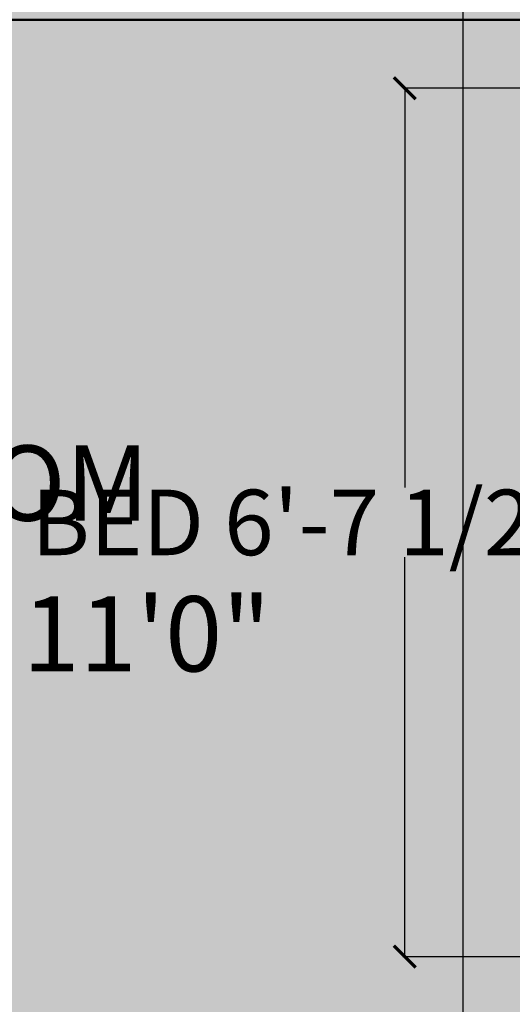
# Model space of a CAD drawing. Units: inches. Extents: x 528 to 2620, y -1066 to 798.
# Tile 27 of 41: x 1112 to 1157, y 620 to 710. Entities that reach past the tile are written whole.
import ezdxf

# ---------------------------------------------------------------- set-up
doc = ezdxf.new("R2010")
doc.units = ezdxf.units.IN
doc.header["$MEASUREMENT"] = 0
for name, color, linetype, lineweight in [('A-ANNO-DIMS', 2, 'Continuous', 18), ('A-AREA-IDEN', 7, 'Continuous', 18), ('A-WALL', 7, 'Continuous', 50), ('A-WALL-PATT', 8, 'Continuous', 13)]:
    doc.layers.add(name, color=color, linetype=linetype, lineweight=lineweight)
doc.styles.get("Standard").update_dxf_attribs({"font": 'arial.ttf'})
doc.dimstyles.get("Standard").update_dxf_attribs({"dimtxt": 6, "dimasz": 2, "dimexe": 0.18, "dimexo": 0.0625, "dimgap": 0.09, "dimtad": 0, "dimtih": 1, "dimtoh": 1, "dimdec": 1, "dimzin": 0, "dimdsep": 46, "dimlunit": 3, "dimtxsty": 'Standard', "dimblk": 'ARCHTICK', "dimcen": 0.09, "dimadec": 0, "dimazin": 0, "dimtfac": 1, "dimtdec": 1, "dimtofl": 0, "dimtmove": 0, "dimatfit": 3, "dimfxl": 1, "dimtolj": 1, "dimtzin": 0, "dimarcsym": 0})

# ---------------------------------------------------------------- blocks, each defined once
blk = doc.blocks.new('_ArchTick')
at = {"color": 0, "linetype": 'ByBlock', "const_width": 0.15}
blk.add_lwpolyline([(-0.5, -0.5), (0.5, 0.5)], dxfattribs=at)
blk = doc.blocks.new('*D42')
at = {"layer": 'A-ANNO-DIMS', "color": 0, "lineweight": -2, "transparency": 16777216}
for p, q in [((1159.521, 703.64), (1147.464, 703.64)), ((1147.644, 703.64), (1147.644, 667.032)), ((1147.644, 624.039), (1147.644, 660.647)), ((1159.521, 624.039), (1147.464, 624.039))]:
    blk.add_line(p, q, dxfattribs=at)
at = {"layer": 'Defpoints', "color": 0, "transparency": 16777216}
for p in [(1159.584, 703.64), (1147.644, 624.039), (1159.584, 624.039)]:
    blk.add_point(p, dxfattribs=at)
at = {"layer": 'A-ANNO-DIMS', "color": 0, "lineweight": -2, "transparency": 16777216, "xscale": 2, "yscale": 2, "zscale": 2}
for p, rotation in [((1147.644, 703.64), 90), ((1147.644, 624.039), 270)]:
    blk.add_blockref('_ArchTick', p, dxfattribs=dict(at, rotation=rotation))
at = {"layer": 'A-ANNO-DIMS', "color": 0, "transparency": 16777216, "insert": (1147.644, 663.839), "char_height": 6, "attachment_point": 5}
blk.add_mtext('\\A1;BED 6\'-7 1/2" TYP.', dxfattribs=at)
blk = doc.blocks.new('*D66')
at = {"layer": 'A-ANNO-DIMS', "color": 0, "lineweight": -2, "transparency": 16777216}
for p, q in [((1065.996, 400.485), (1065.996, 751.102)), ((1065.996, 750.922), (1101.456, 750.922)), ((1152.996, 750.922), (1117.537, 750.922)), ((1152.996, 400.485), (1152.996, 751.102))]:
    blk.add_line(p, q, dxfattribs=at)
at = {"layer": 'Defpoints', "color": 0, "transparency": 16777216}
for p in [(1152.996, 750.922), (1065.996, 400.422), (1152.996, 400.422)]:
    blk.add_point(p, dxfattribs=at)
at = {"layer": 'A-ANNO-DIMS', "color": 0, "lineweight": -2, "transparency": 16777216, "xscale": 2, "yscale": 2, "zscale": 2, "rotation": 180}
blk.add_blockref('_ArchTick', (1065.996, 750.922), dxfattribs=at)
at = {"layer": 'A-ANNO-DIMS', "color": 0, "lineweight": -2, "transparency": 16777216, "xscale": 2, "yscale": 2, "zscale": 2}
blk.add_blockref('_ArchTick', (1152.996, 750.922), dxfattribs=at)
at = {"layer": 'A-ANNO-DIMS', "color": 0, "transparency": 16777216, "insert": (1109.496, 750.922), "char_height": 6, "attachment_point": 5}
blk.add_mtext('\\A1;7\'-3"', dxfattribs=at)

msp = doc.modelspace()

# ---------------------------------------------------------------- hatches: boundary and pattern name
at = {"layer": 'A-WALL-PATT', "transparency": 33554521}
h = msp.add_hatch(color=256, dxfattribs=at)
h.dxf.hatch_style = 1
h.paths.add_polyline_path([(1065.996, 709.922), (1114.496, 709.922), (1114.496, 718.922), (1056.996, 718.922), (1056.996, 667.922), (1065.996, 667.922)])
h.paths.add_polyline_path([(1227.496, 718.922), (1162.496, 718.922), (1162.496, 709.922), (1210.996, 709.922), (1210.996, 577.922), (1205.418, 577.922), (1205.496, 573.422), (1210.996, 573.422), (1210.996, 567.422), (1215.496, 567.422), (1215.496, 669.422), (1267.996, 669.422), (1267.996, 675.922), (1263.496, 675.922), (1263.496, 673.922), (1215.496, 673.922), (1215.496, 709.922), (1227.496, 709.922)])
h.paths.add_polyline_path([(1344.996, 718.922), (1315.996, 718.922), (1315.996, 709.922), (1335.996, 709.922), (1335.996, 641.672), (1344.996, 641.672)])
h.paths.add_polyline_path([(1065.996, 619.922), (1056.996, 619.922), (1056.996, 561.422), (1065.996, 561.422), (1065.996, 573.422), (1160.996, 573.422), (1160.996, 569.422), (1165.496, 569.422), (1165.496, 577.922), (1065.996, 577.922)])
h.paths.add_polyline_path([(1215.996, 391.422), (1215.996, 400.422), (1206.996, 400.422), (1200.996, 400.422), (1200.996, 397.422), (1200.996, 391.422), (1206.996, 391.422), (1206.996, 268.922), (1251.996, 268.922), (1251.996, 277.922), (1215.996, 277.922), (1215.996, 359.767)])
h.paths.add_polyline_path([(1344.996, 395.922), (1335.996, 395.922), (1287.996, 395.922), (1287.996, 391.422), (1335.996, 391.422), (1335.996, 277.922), (1299.996, 277.922), (1299.996, 268.922), (1344.996, 268.922)])
h.paths.add_polyline_path([(1344.996, 593.672), (1335.996, 593.672), (1335.996, 525.422), (1215.496, 525.422), (1215.496, 527.172), (1210.996, 527.172), (1210.996, 520.922), (1335.996, 520.922), (1335.996, 443.922), (1344.996, 443.922)])
h.paths.add_polyline_path([(1065.996, 520.922), (1165.496, 520.922), (1165.496, 545.422), (1160.996, 545.422), (1160.996, 525.422), (1065.996, 525.422), (1065.996, 537.422), (1056.996, 537.422), (1056.996, 484.672), (1065.996, 484.672)])
h.paths.add_polyline_path([(1065.996, 436.672), (1056.996, 436.672), (1056.996, 391.422), (1085.496, 391.422), (1085.496, 400.422), (1065.996, 400.422)])
h.paths.add_polyline_path([(1152.996, 397.422), (1152.996, 400.422), (1133.496, 400.422), (1133.496, 391.422), (1152.996, 391.422)])
at = {"layer": 'A-WALL-PATT', "transparency": 33554681}
h = msp.add_hatch(color=256, dxfattribs=at)
h.dxf.hatch_style = 1
h.paths.add_polyline_path([(1061.996, 665.922), (1060.996, 665.922), (1060.996, 621.922), (1061.996, 621.922)])
h.paths.add_polyline_path([(1065.996, 667.922), (1056.996, 667.922), (1056.996, 665.922), (1065.996, 665.922)])
h.paths.add_polyline_path([(1065.996, 621.922), (1056.996, 621.922), (1056.996, 619.922), (1065.996, 619.922)])
h.paths.add_polyline_path([(1160.496, 714.922), (1116.496, 714.922), (1116.496, 713.922), (1160.496, 713.922)])
h.paths.add_polyline_path([(1162.496, 718.922), (1160.496, 718.922), (1160.496, 709.922), (1162.496, 709.922)])
h.paths.add_polyline_path([(1116.496, 718.922), (1114.496, 718.922), (1114.496, 709.922), (1116.496, 709.922)])
h.paths.add_polyline_path([(1251.496, 714.922), (1227.496, 714.922), (1227.496, 713.922), (1251.496, 713.922)])
h.paths.add_polyline_path([(1313.996, 714.922), (1269.996, 714.922), (1269.996, 713.922), (1313.996, 713.922)])
h.paths.add_polyline_path([(1315.996, 718.922), (1313.996, 718.922), (1313.996, 709.922), (1315.996, 709.922)])
h.paths.add_polyline_path([(1269.996, 718.922), (1267.996, 718.922), (1267.996, 709.922), (1269.996, 709.922)])
h.paths.add_polyline_path([(1087.496, 400.422), (1085.496, 400.422), (1085.496, 391.422), (1087.496, 391.422)])
h.paths.add_polyline_path([(1131.496, 396.422), (1087.496, 396.422), (1087.496, 395.422), (1131.496, 395.422)])
h.paths.add_polyline_path([(1133.496, 400.422), (1131.496, 400.422), (1131.496, 391.422), (1133.496, 391.422)])
h.paths.add_polyline_path([(1065.996, 438.672), (1056.996, 438.672), (1056.996, 436.672), (1065.996, 436.672)])
h.paths.add_polyline_path([(1065.996, 484.672), (1056.996, 484.672), (1056.996, 482.672), (1065.996, 482.672)])
h.paths.add_polyline_path([(1061.996, 482.672), (1060.996, 482.672), (1060.996, 438.672), (1061.996, 438.672)])
h = msp.add_hatch(color=256, dxfattribs=at)
h.dxf.hatch_style = 1
h.paths.add_polyline_path([(1065.996, 665.922), (1061.996, 665.922), (1061.996, 621.922), (1065.996, 621.922)])
h.paths.add_polyline_path([(1060.996, 665.922), (1056.996, 665.922), (1056.996, 621.922), (1060.996, 621.922)])
h.paths.add_polyline_path([(1160.496, 713.922), (1116.496, 713.922), (1116.496, 709.922), (1160.496, 709.922)])
h.paths.add_polyline_path([(1160.496, 718.922), (1116.496, 718.922), (1116.496, 714.922), (1160.496, 714.922)])
h.paths.add_polyline_path([(1251.496, 713.922), (1227.496, 713.922), (1227.496, 709.922), (1251.496, 709.922)])
h.paths.add_polyline_path([(1251.496, 718.922), (1227.496, 718.922), (1227.496, 714.922), (1251.496, 714.922)])
h.paths.add_polyline_path([(1313.996, 713.922), (1269.996, 713.922), (1269.996, 709.922), (1313.996, 709.922)])
h.paths.add_polyline_path([(1313.996, 718.922), (1269.996, 718.922), (1269.996, 714.922), (1313.996, 714.922)])
h.paths.add_polyline_path([(1344.996, 639.672), (1340.996, 639.672), (1340.996, 595.672), (1344.996, 595.672)])
h.paths.add_polyline_path([(1339.996, 639.672), (1335.996, 639.672), (1335.996, 595.672), (1339.996, 595.672)])
h.paths.add_polyline_path([(1344.996, 441.922), (1340.996, 441.922), (1340.996, 397.922), (1344.996, 397.922)])
h.paths.add_polyline_path([(1339.996, 441.922), (1335.996, 441.922), (1335.996, 397.922), (1339.996, 397.922)])
h.paths.add_polyline_path([(1297.996, 272.922), (1253.996, 272.922), (1253.996, 268.922), (1297.996, 268.922)])
h.paths.add_polyline_path([(1297.996, 277.922), (1253.996, 277.922), (1253.996, 273.922), (1297.996, 273.922)])
h.paths.add_polyline_path([(1131.496, 395.422), (1087.496, 395.422), (1087.496, 391.422), (1131.496, 391.422)])
h.paths.add_polyline_path([(1131.496, 400.422), (1087.496, 400.422), (1087.496, 396.422), (1131.496, 396.422)])
h.paths.add_polyline_path([(1065.996, 482.672), (1061.996, 482.672), (1061.996, 438.672), (1065.996, 438.672)])
h.paths.add_polyline_path([(1060.996, 482.672), (1056.996, 482.672), (1056.996, 438.672), (1060.996, 438.672)])
h.paths.add_polyline_path([(1065.996, 561.422), (1061.996, 561.422), (1061.996, 537.422), (1065.996, 537.422)])
h.paths.add_polyline_path([(1060.996, 561.422), (1056.996, 561.422), (1056.996, 537.422), (1060.996, 537.422)])
at = {"layer": 'A-WALL-PATT', "transparency": 33554536}
h = msp.add_hatch(color=256, dxfattribs=at)
h.dxf.hatch_style = 1
h.paths.add_polyline_path([(1335.996, 709.922), (1267.996, 709.922), (1267.996, 699.922), (1266.746, 699.922), (1266.746, 675.922), (1267.996, 675.922), (1267.996, 669.422), (1215.496, 669.422), (1215.496, 567.172), (1216.996, 567.172), (1256.996, 567.172), (1256.996, 565.422), (1256.958, 565.422, -0.401453), (1216.996, 527.172), (1215.496, 527.172), (1215.496, 525.422), (1335.996, 525.422)], flags=17)
h.paths.add_polyline_path([(1285.032, 635.927), (1285.229, 636.128), (1285.672, 636.263), (1286.206, 636.02), (1286.976, 636.084), (1332.983, 636.084), (1333.363, 636.222), (1333.82, 636.084), (1334.115, 635.714), (1334.115, 635.3), (1333.907, 634.86), (1333.82, 634.827), (1333.82, 592.738), (1333.967, 592.604), (1334.115, 592.291), (1334.115, 591.877), (1333.82, 591.507), (1333.363, 591.369), (1332.983, 591.507), (1332.638, 591.789), (1332.638, 591.507), (1286.976, 591.507), (1286.173, 591.672), (1286.066, 591.574), (1285.681, 591.37), (1285.229, 591.507), (1285.032, 591.709), (1284.834, 592.098), (1284.983, 592.537), (1285.13, 592.688), (1285.13, 634.948), (1284.983, 635.099), (1284.834, 635.537)], flags=16)
h.paths.add_polyline_path([(1285.032, 635.927), (1285.229, 636.128), (1285.672, 636.263), (1286.206, 636.02), (1286.976, 636.084), (1332.983, 636.084), (1333.363, 636.222), (1333.82, 636.084), (1334.115, 635.714), (1334.115, 635.3), (1333.967, 634.987), (1333.82, 634.853), (1333.82, 592.738), (1333.967, 592.604), (1334.115, 592.291), (1334.115, 591.877), (1333.82, 591.507), (1333.363, 591.369), (1332.983, 591.507), (1332.638, 591.789), (1332.638, 592.246), (1332.638, 635.345), (1332.638, 635.802), (1332.983, 636.084), (1312.232, 636.084), (1311.1, 635.479), (1310.632, 635.479), (1310.435, 635.233), (1309.943, 635.099), (1309.696, 634.987), (1309.056, 634.763), (1308.712, 634.607), (1308.318, 634.607), (1307.752, 634.36), (1307.112, 634.271), (1307.013, 634.114), (1306.767, 634.025), (1307.255, 633.283), (1306.866, 633.04), (1306.767, 632.884), (1306.373, 632.637), (1306.029, 632.548), (1305.536, 632.414), (1315.472, 618.494), (1316.321, 619.388), (1312.773, 622.858), (1319.616, 630.109), (1320.067, 629.676), (1320.109, 629.997), (1320.281, 630.601), (1320.527, 631.183), (1320.527, 632.011), (1320.256, 632.548), (1320.109, 633.13), (1320.06, 633.734), (1320.626, 634.025), (1321.216, 634.159), (1321.856, 634.114), (1322.447, 633.913), (1322.989, 633.622), (1324.096, 633.622), (1324.638, 633.913), (1325.229, 634.07), (1325.869, 634.07), (1326.435, 633.913), (1326.976, 633.622), (1328.355, 633.622), (1328.896, 633.913), (1329.487, 634.114), (1330.103, 634.159), (1330.693, 634.025), (1331.284, 633.734), (1331.235, 633.13), (1331.087, 632.548), (1330.792, 632.011), (1330.792, 631.183), (1331.038, 630.601), (1331.235, 629.997), (1331.284, 629.415), (1331.186, 628.788), (1331.038, 628.184), (1330.792, 627.602), (1330.792, 626.774), (1331.038, 626.193), (1331.235, 625.588), (1331.284, 625.007), (1331.186, 624.38), (1331.038, 623.776), (1330.792, 623.239), (1330.792, 622.366), (1331.038, 621.829), (1331.235, 621.247), (1331.284, 620.598), (1331.186, 619.972), (1331.038, 619.367), (1330.792, 618.83), (1330.792, 617.958), (1331.087, 617.421), (1331.235, 616.884), (1331.284, 616.235), (1331.284, 615.518), (1330.693, 615.272), (1330.103, 615.116), (1329.487, 615.116), (1328.896, 615.317), (1328.355, 615.653), (1326.976, 615.653), (1326.435, 615.317), (1325.869, 615.16), (1325.229, 615.16), (1324.638, 615.317), (1324.096, 615.653), (1323.242, 615.653), (1324.933, 614.042), (1322.978, 611.983), (1324.096, 611.983), (1324.638, 612.274), (1325.278, 612.43), (1325.869, 612.43), (1326.484, 612.274), (1327.026, 611.983), (1328.355, 611.983), (1328.896, 612.274), (1329.487, 612.475), (1330.103, 612.52), (1330.743, 612.386), (1331.284, 612.072), (1331.284, 611.356), (1331.284, 610.752), (1331.087, 610.17), (1330.792, 609.633), (1330.792, 608.805), (1331.087, 608.223), (1331.235, 607.619), (1331.284, 606.993), (1331.235, 606.411), (1331.087, 605.807), (1330.792, 605.225), (1330.792, 604.397), (1331.087, 603.815), (1331.235, 603.211), (1331.284, 602.629), (1331.235, 602.002), (1331.087, 601.398), (1330.792, 600.861), (1330.792, 599.988), (1331.087, 599.451), (1331.235, 598.87), (1331.284, 598.221), (1331.235, 597.594), (1331.087, 596.99), (1330.792, 596.453), (1330.792, 595.58), (1331.087, 595.043), (1331.284, 594.506), (1331.284, 593.857), (1330.743, 593.611), (1330.103, 593.477), (1329.487, 593.477), (1328.896, 593.678), (1328.355, 594.014), (1327.026, 594.014), (1326.484, 593.678), (1325.869, 593.521), (1325.278, 593.521), (1324.638, 593.678), (1324.096, 594.014), (1323.038, 594.014), (1322.496, 593.678), (1321.906, 593.477), (1321.266, 593.477), (1320.626, 593.611), (1320.109, 593.857), (1320.109, 594.506), (1320.281, 595.043), (1320.576, 595.58), (1320.576, 596.453), (1320.281, 596.99), (1320.158, 597.594), (1320.104, 598.015), (1319.616, 597.549), (1315.659, 601.729), (1312.232, 591.574), (1311.74, 591.664), (1311.592, 591.91), (1310.78, 592.402), (1309.549, 592.895), (1308.958, 592.895), (1308.712, 593.029), (1308.564, 593.141), (1307.752, 593.521), (1306.767, 593.611), (1307.248, 594.356), (1306.866, 594.595), (1306.373, 594.842), (1306.029, 595.088), (1305.536, 595.244), (1315.465, 609.354), (1310.927, 613.706), (1315.472, 618.494), (1305.536, 632.414), (1306.029, 632.548), (1306.373, 632.637), (1306.767, 632.884), (1306.866, 633.04), (1307.255, 633.283), (1306.767, 634.025), (1307.013, 634.114), (1307.112, 634.271), (1307.752, 634.36), (1308.318, 634.607), (1308.712, 634.607), (1309.056, 634.763), (1309.696, 634.987), (1309.943, 635.099), (1310.435, 635.233), (1310.632, 635.479), (1311.1, 635.479), (1312.232, 636.084), (1286.976, 636.084), (1286.216, 636.021), (1286.411, 635.444), (1286.213, 635.054), (1286.016, 634.853), (1285.869, 634.808), (1285.869, 592.839), (1286.153, 592.731), (1286.41, 592.188), (1286.231, 591.66), (1286.173, 591.672), (1286.066, 591.574), (1285.681, 591.37), (1285.229, 591.507), (1285.032, 591.709), (1284.834, 592.098), (1284.983, 592.537), (1285.13, 592.688), (1285.13, 634.948), (1284.983, 635.099), (1284.834, 635.537)], flags=0)
h.paths.add_polyline_path([(1322.501, 653.596), (1333.646, 653.596), (1333.646, 637.994), (1322.501, 637.994)], flags=16)
h.paths.add_polyline_path([(1323.616, 652.482), (1332.531, 652.482), (1332.531, 639.108), (1323.616, 639.108)], flags=0)
edge = h.paths.add_edge_path(flags=0)
edge.add_ellipse((1328.073, 645.795), major_axis=(2.245, 2.245), ratio=1, start_angle=405, end_angle=495, ccw=False)
edge.add_ellipse((1328.073, 645.795), major_axis=(2.245, 2.245), ratio=1, start_angle=675, end_angle=765, ccw=False)
edge.add_ellipse((1328.073, 645.795), major_axis=(2.245, 2.245), ratio=1, start_angle=585, end_angle=675, ccw=False)
edge.add_ellipse((1328.073, 645.795), major_axis=(2.245, 2.245), ratio=1, start_angle=495, end_angle=585, ccw=False)
h.paths.add_polyline_path([(1320.576, 628.386), (1320.33, 628.005), (1320.615, 628.548)], flags=0)
h.paths.add_polyline_path([(1317.893, 604.889), (1318.78, 604.643), (1319.764, 604.285), (1318.878, 604.531)], flags=0)
h.paths.add_polyline_path([(1320.33, 599.653), (1320.576, 599.25), (1320.576, 599.16)], flags=0)
h.paths.add_polyline_path([(1322.501, 589.597), (1333.646, 589.597), (1333.646, 573.995), (1322.501, 573.995)], flags=16)
h.paths.add_polyline_path([(1323.616, 588.482), (1332.531, 588.482), (1332.531, 575.109), (1323.616, 575.109)], flags=0)
edge = h.paths.add_edge_path(flags=0)
edge.add_ellipse((1328.073, 581.796), major_axis=(-2.245, 2.245), ratio=1, start_angle=-45, end_angle=45, ccw=False)
edge.add_ellipse((1328.073, 581.796), major_axis=(-2.245, 2.245), ratio=1, start_angle=-135, end_angle=-45, ccw=False)
edge.add_ellipse((1328.073, 581.796), major_axis=(-2.245, 2.245), ratio=1, start_angle=135, end_angle=-135, ccw=False)
edge.add_ellipse((1328.073, 581.796), major_axis=(-2.245, 2.245), ratio=1, start_angle=45, end_angle=135, ccw=False)
h.paths.add_polyline_path([(1264.746, 699.922), (1263.496, 699.922), (1263.496, 709.922), (1215.496, 709.922), (1215.496, 673.922), (1263.496, 673.922), (1263.496, 675.922), (1264.746, 675.922)], flags=16)
h.paths.add_polyline_path([(1162.192, 569.422), (1160.996, 569.422), (1160.996, 573.422), (1065.996, 573.422), (1065.996, 525.422), (1160.996, 525.422), (1160.996, 545.422), (1162.192, 545.422)])
h.paths.add_polyline_path([(1256.958, 565.422), (1256.996, 565.422), (1256.996, 567.172), (1216.996, 567.172), (1215.496, 567.172), (1215.496, 567.422), (1210.996, 567.422), (1210.996, 573.422), (1205.496, 573.422), (1205.418, 577.922), (1210.996, 577.922), (1210.996, 709.922), (1065.996, 709.922), (1065.996, 577.922), (1165.496, 577.922), (1165.496, 569.422), (1164.192, 569.422), (1164.192, 545.422), (1165.496, 545.422), (1165.496, 520.922), (1152.996, 520.922), (1152.996, 484.922), (1101.996, 484.922), (1101.996, 436.422), (1152.996, 436.422), (1152.996, 400.422), (1152.996, 391.422), (1200.996, 391.422), (1200.996, 400.422), (1206.996, 400.422), (1215.996, 400.422), (1215.996, 391.422), (1215.996, 277.922), (1335.996, 277.922), (1335.996, 391.422), (1287.996, 391.422), (1287.996, 395.922), (1335.996, 395.922), (1335.996, 443.922), (1335.996, 520.922), (1210.996, 520.922), (1210.996, 527.172), (1215.496, 527.172), (1216.996, 527.172, 0.401453)])
h.paths.add_polyline_path([(1167.246, 579.422), (1165.496, 579.422), (1165.496, 619.422), (1167.246, 619.422)], flags=16)
h.paths.add_polyline_path([(1227.97, 501.564), (1236.36, 502.031), (1236.36, 492.555), (1227.97, 493.021, -0.254069)], flags=16)
h.paths.add_polyline_path([(1243.336, 515.692, -0.254069), (1251.879, 515.692), (1252.345, 507.301), (1242.87, 507.301)], flags=16)
h.paths.add_polyline_path([(1239.185, 504.685), (1256.03, 504.685), (1256.03, 479.416), (1239.185, 479.416)], flags=16)
h.paths.add_polyline_path([(1227.97, 489.602), (1236.36, 490.068), (1236.36, 480.592), (1227.97, 481.058, -0.254069)], flags=16)
h.paths.add_polyline_path([(1197.201, 624.039), (1197.201, 639.641), (1208.345, 639.641), (1208.345, 624.039)], flags=16)
h.paths.add_polyline_path([(1198.315, 625.153), (1198.315, 638.526), (1207.231, 638.526), (1207.231, 625.153)], flags=0)
h.paths.add_polyline_path([(1258.855, 502.031), (1267.245, 501.564, -0.254069), (1267.245, 493.021), (1258.855, 492.555)], flags=16)
h.paths.add_polyline_path([(1271.589, 519.657), (1333.671, 519.657), (1333.671, 451.595), (1319.087, 451.595), (1319.087, 505.072), (1288.093, 505.072), (1284.447, 505.072, -0.883215), (1270.678, 514.188), (1270.678, 518.745, -0.414214)], flags=16)
h.paths.add_polyline_path([(1331.848, 517.834), (1331.848, 453.418), (1328.202, 453.418), (1328.202, 505.072), (1298.424, 505.072), (1298.424, 514.188), (1288.093, 514.188), (1288.093, 517.834)], flags=0)
h.paths.add_polyline_path([(1242.87, 476.8), (1252.345, 476.8), (1251.879, 468.409, -0.254069), (1243.336, 468.409)], flags=16)
h.paths.add_polyline_path([(1258.855, 490.068), (1267.245, 489.602, -0.254069), (1267.245, 481.058), (1258.855, 480.592)], flags=16)
h.paths.add_polyline_path([(1161.676, 641.551), (1160.873, 641.716), (1160.765, 641.618), (1160.38, 641.414), (1159.928, 641.551), (1159.731, 641.753), (1159.534, 642.142), (1159.682, 642.581), (1159.83, 642.732), (1159.83, 684.992), (1159.682, 685.143), (1159.534, 685.582), (1159.731, 685.971), (1159.928, 686.172), (1160.371, 686.307), (1160.905, 686.064), (1161.676, 686.128), (1207.682, 686.128), (1208.063, 686.266), (1208.519, 686.128), (1208.815, 685.758), (1208.815, 685.344), (1208.607, 684.904), (1208.519, 684.871), (1208.519, 642.782), (1208.667, 642.648), (1208.877, 642.201), (1208.716, 641.797), (1208.519, 641.551), (1208.063, 641.413), (1207.682, 641.551), (1207.338, 641.833), (1207.338, 641.551)], flags=16)
h.paths.add_polyline_path([(1186.931, 641.618), (1186.439, 641.708), (1186.291, 641.954), (1185.479, 642.446), (1184.248, 642.939), (1183.658, 642.939), (1183.411, 643.073), (1183.264, 643.185), (1182.451, 643.565), (1181.467, 643.655), (1181.948, 644.4), (1181.565, 644.639), (1181.073, 644.886), (1180.728, 645.132), (1180.236, 645.288), (1190.164, 659.398), (1185.627, 663.75), (1190.171, 668.538), (1180.236, 682.458), (1180.728, 682.592), (1181.073, 682.681), (1181.467, 682.928), (1181.565, 683.084), (1181.954, 683.327), (1181.467, 684.069), (1181.713, 684.158), (1181.811, 684.315), (1182.451, 684.404), (1183.018, 684.651), (1183.411, 684.651), (1183.756, 684.807), (1184.396, 685.031), (1184.642, 685.143), (1185.135, 685.277), (1185.331, 685.523), (1185.799, 685.523), (1186.931, 686.128), (1161.676, 686.128), (1160.915, 686.065), (1161.111, 685.488), (1160.913, 685.098), (1160.716, 684.897), (1160.568, 684.852), (1160.568, 642.883), (1160.853, 642.775), (1161.109, 642.232), (1160.931, 641.704), (1160.873, 641.716), (1160.765, 641.618), (1160.38, 641.414), (1159.928, 641.551), (1159.731, 641.753), (1159.534, 642.142), (1159.682, 642.581), (1159.83, 642.732), (1159.83, 684.992), (1159.682, 685.143), (1159.534, 685.582), (1159.731, 685.971), (1159.928, 686.172), (1160.371, 686.307), (1160.905, 686.064), (1161.676, 686.128), (1207.682, 686.128), (1208.063, 686.266), (1208.519, 686.128), (1208.815, 685.758), (1208.815, 685.344), (1208.667, 685.031), (1208.519, 684.897), (1208.519, 642.782), (1208.667, 642.648), (1208.877, 642.201), (1208.716, 641.797), (1208.519, 641.551), (1208.063, 641.413), (1207.682, 641.551), (1207.338, 641.833), (1207.338, 642.29), (1207.338, 685.389), (1207.338, 685.846), (1207.682, 686.128), (1186.931, 686.128), (1185.799, 685.523), (1185.331, 685.523), (1185.135, 685.277), (1184.642, 685.143), (1184.396, 685.031), (1183.756, 684.807), (1183.411, 684.651), (1183.018, 684.651), (1182.451, 684.404), (1181.811, 684.315), (1181.713, 684.158), (1181.467, 684.069), (1181.954, 683.327), (1181.565, 683.084), (1181.467, 682.928), (1181.073, 682.681), (1180.728, 682.592), (1180.236, 682.458), (1190.171, 668.538), (1191.021, 669.432), (1187.473, 672.902), (1194.316, 680.153), (1194.767, 679.72), (1194.808, 680.041), (1194.981, 680.645), (1195.227, 681.227), (1195.227, 682.055), (1194.956, 682.592), (1194.808, 683.174), (1194.759, 683.778), (1195.325, 684.069), (1195.916, 684.203), (1196.556, 684.158), (1197.147, 683.957), (1197.688, 683.666), (1198.796, 683.666), (1199.338, 683.957), (1199.928, 684.114), (1200.568, 684.114), (1201.135, 683.957), (1201.676, 683.666), (1203.055, 683.666), (1203.596, 683.957), (1204.187, 684.158), (1204.802, 684.203), (1205.393, 684.069), (1205.984, 683.778), (1205.935, 683.174), (1205.787, 682.592), (1205.491, 682.055), (1205.491, 681.227), (1205.738, 680.645), (1205.935, 680.041), (1205.984, 679.459), (1205.885, 678.832), (1205.738, 678.228), (1205.491, 677.646), (1205.491, 676.818), (1205.738, 676.237), (1205.935, 675.632), (1205.984, 675.051), (1205.885, 674.424), (1205.738, 673.82), (1205.491, 673.283), (1205.491, 672.41), (1205.738, 671.873), (1205.935, 671.291), (1205.984, 670.642), (1205.885, 670.016), (1205.738, 669.411), (1205.491, 668.874), (1205.491, 668.002), (1205.787, 667.465), (1205.935, 666.928), (1205.984, 666.279), (1205.984, 665.563), (1205.393, 665.316), (1204.802, 665.16), (1204.187, 665.16), (1203.596, 665.361), (1203.055, 665.697), (1201.676, 665.697), (1201.135, 665.361), (1200.568, 665.204), (1199.928, 665.204), (1199.338, 665.361), (1198.796, 665.697), (1197.942, 665.697), (1199.633, 664.086), (1197.678, 662.027), (1198.796, 662.027), (1199.338, 662.318), (1199.978, 662.474), (1200.568, 662.474), (1201.184, 662.318), (1201.725, 662.027), (1203.055, 662.027), (1203.596, 662.318), (1204.187, 662.519), (1204.802, 662.564), (1205.442, 662.43), (1205.984, 662.116), (1205.984, 661.4), (1205.984, 660.796), (1205.787, 660.214), (1205.491, 659.677), (1205.491, 658.849), (1205.787, 658.267), (1205.935, 657.663), (1205.984, 657.037), (1205.935, 656.455), (1205.787, 655.851), (1205.491, 655.269), (1205.491, 654.441), (1205.787, 653.859), (1205.935, 653.255), (1205.984, 652.673), (1205.935, 652.046), (1205.787, 651.442), (1205.491, 650.905), (1205.491, 650.032), (1205.787, 649.495), (1205.935, 648.914), (1205.984, 648.265), (1205.935, 647.638), (1205.787, 647.034), (1205.491, 646.497), (1205.491, 645.624), (1205.787, 645.087), (1205.984, 644.55), (1205.984, 643.901), (1205.442, 643.655), (1204.802, 643.521), (1204.187, 643.521), (1203.596, 643.722), (1203.055, 644.058), (1201.725, 644.058), (1201.184, 643.722), (1200.568, 643.565), (1199.978, 643.565), (1199.338, 643.722), (1198.796, 644.058), (1197.738, 644.058), (1197.196, 643.722), (1196.605, 643.521), (1195.965, 643.521), (1195.325, 643.655), (1194.808, 643.901), (1194.808, 644.55), (1194.981, 645.087), (1195.276, 645.624), (1195.276, 646.497), (1194.981, 647.034), (1194.858, 647.638), (1194.803, 648.059), (1194.316, 647.593), (1190.359, 651.773)], flags=16)
h.paths.add_polyline_path([(1195.276, 649.204), (1195.03, 649.697), (1195.276, 649.294)], flags=0)
h.paths.add_polyline_path([(1194.464, 654.329), (1193.578, 654.575), (1192.593, 654.933), (1193.479, 654.687)], flags=0)
h.paths.add_polyline_path([(1195.276, 678.43), (1195.03, 678.049), (1195.314, 678.592)], flags=0)
h.paths.add_polyline_path([(1197.201, 688.038), (1197.201, 703.64), (1208.345, 703.64), (1208.345, 688.038)], flags=16)
h.paths.add_polyline_path([(1198.315, 689.152), (1198.315, 702.526), (1207.231, 702.526), (1207.231, 689.152)], flags=0)
h.paths.add_polyline_path([(1217.099, 329.02), (1230.651, 329.02), (1230.651, 315.468), (1217.099, 315.468)], flags=16)
h.paths.add_polyline_path([(1223.875, 322.244), (1227.263, 322.244), (1227.263, 321.322, -0.414214), (1229.729, 318.856, -1), (1224.797, 318.856), (1223.875, 318.856)], flags=0)
h.paths.add_polyline_path([(1222.115, 325.632, -1), (1218.859, 325.632, -1)], flags=0)
h.paths.add_polyline_path([(1228.25, 325.632, -1), (1226.276, 325.632, -1)], flags=0)
h.paths.add_polyline_path([(1221.533, 318.856, -1), (1219.441, 318.856, -1)], flags=0)
h.paths.add_polyline_path([(1299.145, 293.732), (1299.145, 278.539), (1271.232, 278.539), (1271.232, 293.732)], flags=16)
h.paths.add_polyline_path([(1259.687, 292.213), (1270.624, 292.213, -1), (1270.624, 291.605), (1259.687, 291.605, -1)], flags=16)
h.paths.add_polyline_path([(1259.687, 291.301), (1270.624, 291.301, -1), (1270.624, 290.693), (1259.687, 290.693, -1)], flags=16)
h.paths.add_polyline_path([(1259.687, 290.389), (1270.624, 290.389, -1), (1270.624, 289.782), (1259.687, 289.782, -1)], flags=16)
h.paths.add_polyline_path([(1259.687, 289.478), (1270.624, 289.478, -1), (1270.624, 288.87), (1259.687, 288.87, -1)], flags=16)
h.paths.add_polyline_path([(1259.687, 288.566), (1270.624, 288.566, -1), (1270.624, 287.958), (1259.687, 287.958, -1)], flags=16)
h.paths.add_polyline_path([(1274.406, 292.381), (1283.251, 292.381, -0.414214), (1285.074, 290.558), (1285.074, 283.642, -0.414214), (1283.251, 281.819), (1277.723, 281.819), (1278.673, 280.869, -0.57735), (1279.382, 280.16), (1279.436, 280.106, -1), (1279.027, 279.696), (1278.972, 279.751, -0.57735), (1278.263, 280.46), (1276.904, 281.819), (1274.406, 281.819, -0.414214), (1272.583, 283.642), (1272.583, 290.558, -0.414214)], flags=0)
h.paths.add_polyline_path([(1259.687, 287.655), (1270.624, 287.655, -1), (1270.624, 287.047), (1259.687, 287.047, -1)], flags=16)
h.paths.add_polyline_path([(1259.687, 286.743), (1270.624, 286.743, -1), (1270.624, 286.135), (1259.687, 286.135, -1)], flags=16)
h.paths.add_polyline_path([(1259.687, 285.831), (1270.624, 285.831, -1), (1270.624, 285.224), (1259.687, 285.224, -1)], flags=16)
h.paths.add_polyline_path([(1259.687, 284.92), (1270.624, 284.92, -1), (1270.624, 284.312), (1259.687, 284.312, -1)], flags=16)
h.paths.add_polyline_path([(1259.687, 284.008), (1270.624, 284.008, -1), (1270.624, 283.401), (1259.687, 283.401, -1)], flags=16)
h.paths.add_polyline_path([(1287.823, 292.381), (1296.669, 292.381, -0.414214), (1298.492, 290.558), (1298.492, 283.642, -0.414214), (1296.669, 281.819), (1291.14, 281.819), (1292.09, 280.869, -0.57735), (1292.799, 280.16), (1292.854, 280.106, -1), (1292.445, 279.696), (1292.39, 279.751, -0.57735), (1291.681, 280.46), (1290.322, 281.819), (1287.823, 281.819, -0.414214), (1286, 283.642), (1286, 290.558, -0.414214)], flags=0)
h.paths.add_polyline_path([(1259.687, 283.097), (1270.624, 283.097, -1), (1270.624, 282.489), (1259.687, 282.489, -1)], flags=16)
h.paths.add_polyline_path([(1279.939, 287.607, -1), (1278.01, 287.607, -1)], flags=0)
h.paths.add_polyline_path([(1259.687, 282.185), (1270.624, 282.185, -1), (1270.624, 281.577), (1259.687, 281.577, -1)], flags=16)
h.paths.add_polyline_path([(1259.687, 281.273), (1270.624, 281.273, -1), (1270.624, 280.666), (1259.687, 280.666, -1)], flags=16)
h.paths.add_polyline_path([(1275.156, 284.169, -1), (1274.77, 284.169, -1)], flags=0)
h.paths.add_polyline_path([(1293.357, 287.607, -1), (1291.427, 287.607, -1)], flags=0)
h.paths.add_polyline_path([(1275.144, 280.503), (1276.335, 280.503, -5.828427), (1276.335, 280.117), (1275.144, 280.117, -1)], flags=0)
h.paths.add_polyline_path([(1288.574, 284.169, -1), (1288.188, 284.169, -1)], flags=0)
h.paths.add_polyline_path([(1281.31, 280.503), (1282.501, 280.503, -1), (1282.501, 280.117), (1281.31, 280.117, -5.828427)], flags=0)
h.paths.add_polyline_path([(1288.562, 280.503), (1289.752, 280.503, -5.828427), (1289.752, 280.117), (1288.562, 280.117, -1)], flags=0)
h.paths.add_polyline_path([(1294.727, 280.503), (1295.918, 280.503, -1), (1295.918, 280.117), (1294.727, 280.117, -5.828427)], flags=0)
h.paths.add_polyline_path([(1206.996, 391.422), (1200.996, 391.422), (1061.496, 391.422), (1061.496, 307.96), (1068.996, 307.96), (1068.996, 305.422), (1206.996, 305.422)])
at = {"layer": 'A-WALL-PATT', "transparency": 33554480}
h = msp.add_hatch(color=256, dxfattribs=at)
h.dxf.hatch_style = 1
h.paths.add_polyline_path([(1210.996, 709.922), (1065.996, 709.922), (1065.996, 577.922), (1165.496, 577.922), (1165.496, 579.422), (1165.496, 619.422), (1167.246, 619.422), (1167.246, 619.384, -0.401453), (1205.496, 579.422), (1205.496, 577.922), (1210.996, 577.922)])
h.paths.add_polyline_path([(1160.833, 686.058), (1160.905, 686.064), (1160.765, 686.128)], flags=16)
h.paths.add_polyline_path([(1160.931, 641.704), (1160.931, 641.707), (1160.928, 641.705)], flags=0)
h.paths.add_polyline_path([(1159.83, 684.992), (1159.584, 685.244), (1159.584, 685.82), (1160.016, 686.262), (1160.224, 686.262), (1159.928, 686.172), (1159.731, 685.971), (1159.584, 685.68), (1159.584, 685.434), (1159.682, 685.143), (1159.879, 684.942), (1160.175, 684.807), (1160.421, 684.807), (1160.716, 684.897), (1160.913, 685.098), (1161.111, 685.488), (1161.061, 685.635), (1161.061, 685.249), (1160.568, 684.746), (1160.568, 642.961), (1161.061, 642.514), (1161.061, 641.887), (1160.873, 641.716), (1161.676, 641.551), (1186.533, 641.551), (1186.291, 641.954), (1185.479, 642.446), (1184.248, 642.939), (1183.589, 642.939), (1183.264, 643.185), (1182.451, 643.565), (1181.467, 643.655), (1181.948, 644.4), (1181.565, 644.639), (1181.073, 644.886), (1180.728, 645.132), (1180.236, 645.288), (1190.164, 659.398), (1185.627, 663.75), (1190.171, 668.538), (1180.236, 682.458), (1180.728, 682.592), (1181.073, 682.681), (1181.467, 682.928), (1181.565, 683.084), (1181.954, 683.327), (1181.467, 684.069), (1181.713, 684.158), (1181.811, 684.315), (1182.451, 684.404), (1183.018, 684.651), (1183.411, 684.651), (1183.756, 684.807), (1184.396, 685.031), (1184.642, 685.143), (1185.135, 685.277), (1185.331, 685.523), (1185.799, 685.523), (1186.931, 686.128), (1207.682, 686.128), (1208.063, 686.266), (1208.631, 686.094), (1208.877, 685.478), (1208.607, 684.904), (1208.519, 684.871), (1208.519, 642.782), (1208.815, 642.514), (1208.815, 641.921), (1208.448, 641.462), (1207.792, 641.462), (1207.338, 641.833), (1207.338, 641.551), (1161.676, 641.551), (1160.928, 641.705), (1160.38, 641.414), (1159.816, 641.585), (1159.534, 642.142), (1159.722, 642.699), (1159.83, 642.756)], flags=16)
h.paths.add_polyline_path([(1159.83, 684.992), (1159.584, 685.244), (1159.584, 685.82), (1160.016, 686.262), (1160.224, 686.262), (1159.928, 686.172), (1159.731, 685.971), (1159.584, 685.68), (1159.584, 685.434), (1159.682, 685.143), (1159.83, 684.992), (1159.83, 642.732), (1159.682, 642.581), (1159.584, 642.29), (1159.584, 642.044), (1159.731, 641.753), (1160.016, 641.462), (1160.224, 641.462), (1159.816, 641.585), (1159.534, 642.142), (1159.682, 642.581), (1159.83, 642.732)], flags=0)
h.paths.add_polyline_path([(1207.682, 686.128), (1207.517, 686.128), (1207.488, 686.057)], flags=0)
h.paths.add_polyline_path([(1195.276, 648.712), (1195.287, 648.521), (1195.522, 648.746), (1195.522, 648.802), (1195.276, 649.204)], flags=0)
h.paths.add_polyline_path([(1194.767, 679.72), (1194.808, 680.041), (1194.981, 680.645), (1195.227, 681.227), (1195.227, 682.055), (1194.956, 682.592), (1194.808, 683.174), (1194.759, 683.778), (1195.325, 684.069), (1195.916, 684.203), (1196.556, 684.158), (1197.147, 683.957), (1197.688, 683.666), (1198.796, 683.666), (1199.338, 683.957), (1199.928, 684.114), (1200.568, 684.114), (1201.135, 683.957), (1201.676, 683.666), (1203.055, 683.666), (1203.596, 683.957), (1204.187, 684.158), (1204.802, 684.203), (1205.393, 684.069), (1205.984, 683.778), (1205.935, 683.174), (1205.787, 682.592), (1205.491, 682.055), (1205.491, 681.227), (1205.738, 680.645), (1205.935, 680.041), (1205.984, 679.459), (1205.885, 678.832), (1205.738, 678.228), (1205.491, 677.646), (1205.491, 676.818), (1205.738, 676.237), (1205.935, 675.632), (1205.984, 675.051), (1205.885, 674.424), (1205.738, 673.82), (1205.491, 673.283), (1205.491, 672.41), (1205.738, 671.873), (1205.935, 671.291), (1205.984, 670.642), (1205.885, 670.016), (1205.738, 669.411), (1205.491, 668.874), (1205.491, 668.002), (1205.787, 667.465), (1205.935, 666.928), (1205.984, 666.279), (1205.984, 665.563), (1205.393, 665.316), (1204.802, 665.16), (1204.187, 665.16), (1203.596, 665.361), (1203.055, 665.697), (1201.676, 665.697), (1201.135, 665.361), (1200.568, 665.204), (1199.928, 665.204), (1199.338, 665.361), (1198.796, 665.697), (1197.942, 665.697), (1199.633, 664.086), (1197.678, 662.027), (1198.796, 662.027), (1199.338, 662.318), (1199.978, 662.474), (1200.568, 662.474), (1201.184, 662.318), (1201.725, 662.027), (1203.055, 662.027), (1203.596, 662.318), (1204.187, 662.519), (1204.802, 662.564), (1205.442, 662.43), (1205.984, 662.116), (1205.984, 661.4), (1205.984, 660.796), (1205.787, 660.214), (1205.491, 659.677), (1205.491, 658.849), (1205.787, 658.267), (1205.935, 657.663), (1205.984, 657.037), (1205.935, 656.455), (1205.787, 655.851), (1205.491, 655.269), (1205.491, 654.441), (1205.787, 653.859), (1205.935, 653.255), (1205.984, 652.673), (1205.935, 652.046), (1205.787, 651.442), (1205.491, 650.905), (1205.491, 650.032), (1205.787, 649.495), (1205.935, 648.914), (1205.984, 648.265), (1205.935, 647.638), (1205.787, 647.034), (1205.491, 646.497), (1205.491, 645.624), (1205.787, 645.087), (1205.984, 644.55), (1205.984, 643.901), (1205.442, 643.655), (1204.802, 643.521), (1204.187, 643.521), (1203.596, 643.722), (1203.055, 644.058), (1201.725, 644.058), (1201.184, 643.722), (1200.568, 643.565), (1199.978, 643.565), (1199.338, 643.722), (1198.796, 644.058), (1197.738, 644.058), (1195.522, 644.304), (1205.295, 644.304), (1205.295, 661.445), (1197.125, 661.445), (1199.633, 664.086), (1196.004, 667.543), (1201.479, 673.283), (1195.522, 678.996), (1195.522, 678.922), (1195.31, 678.575), (1195.276, 678.43), (1195.03, 678.049), (1195.276, 678.519), (1195.276, 679.232)], flags=0)
h.paths.add_polyline_path([(1192.593, 654.933), (1193.479, 654.687), (1194.464, 654.329), (1193.578, 654.575)], flags=0)
h.paths.add_polyline_path([(1192.593, 672.79), (1193.43, 673.037), (1194.295, 673.351), (1194.29, 673.358), (1193.578, 673.149)], flags=0)
h.paths.add_polyline_path([(1195.276, 649.294), (1195.03, 649.697), (1195.296, 649.165)], flags=0)
h.paths.add_polyline_path([(1197.201, 639.641), (1208.345, 639.641), (1208.345, 624.039), (1197.201, 624.039)], flags=16)
h.paths.add_polyline_path([(1198.315, 638.526), (1207.231, 638.526), (1207.231, 625.153), (1198.315, 625.153)], flags=0)
edge = h.paths.add_edge_path(flags=0)
edge.add_ellipse((1202.773, 631.84), major_axis=(-2.245, 2.245), ratio=1, start_angle=-45, end_angle=45, ccw=False)
edge.add_ellipse((1202.773, 631.84), major_axis=(-2.245, 2.245), ratio=1, start_angle=-135, end_angle=-45, ccw=False)
edge.add_ellipse((1202.773, 631.84), major_axis=(-2.245, 2.245), ratio=1, start_angle=135, end_angle=-135, ccw=False)
edge.add_ellipse((1202.773, 631.84), major_axis=(-2.245, 2.245), ratio=1, start_angle=45, end_angle=135, ccw=False)
h.paths.add_polyline_path([(1197.201, 688.038), (1197.201, 703.64), (1208.345, 703.64), (1208.345, 688.038)], flags=16)
h.paths.add_polyline_path([(1198.315, 689.152), (1198.315, 702.526), (1207.231, 702.526), (1207.231, 689.152)], flags=0)
edge = h.paths.add_edge_path(flags=0)
edge.add_ellipse((1202.773, 695.839), major_axis=(2.245, 2.245), ratio=1, start_angle=405, end_angle=495, ccw=False)
edge.add_ellipse((1202.773, 695.839), major_axis=(2.245, 2.245), ratio=1, start_angle=675, end_angle=765, ccw=False)
edge.add_ellipse((1202.773, 695.839), major_axis=(2.245, 2.245), ratio=1, start_angle=585, end_angle=675, ccw=False)
edge.add_ellipse((1202.773, 695.839), major_axis=(2.245, 2.245), ratio=1, start_angle=495, end_angle=585, ccw=False)
h.paths.add_polyline_path([(1207.338, 685.389), (1207.338, 685.846), (1207.792, 686.217), (1208.448, 686.217), (1208.815, 685.758), (1208.815, 685.165), (1208.519, 684.897), (1208.519, 642.782), (1208.815, 642.514), (1208.815, 641.921), (1208.448, 641.462), (1207.792, 641.462), (1207.338, 641.833), (1207.338, 642.29)], flags=0)
h.paths.add_polyline_path([(1207.469, 642.678), (1207.989, 643.009), (1208.607, 642.775), (1208.877, 642.201), (1208.631, 641.585), (1208.063, 641.413), (1207.488, 641.622), (1207.284, 642.132)], flags=16)
h.paths.add_polyline_path([(1207.633, 684.897), (1207.879, 684.74), (1208.347, 684.74), (1208.667, 685.031), (1208.815, 685.344), (1208.815, 685.635), (1208.716, 685.881), (1208.448, 686.217), (1208.224, 686.217), (1208.631, 686.094), (1208.877, 685.478), (1208.667, 685.031), (1208.347, 684.74), (1207.786, 684.74)], flags=16)
h.paths.add_polyline_path([(1076.476, 648.31), (1137.071, 648.31), (1137.071, 658.865), (1076.476, 658.865)], flags=24)
h.paths.add_polyline_path([(1076.71, 662.103), (1130.014, 662.103), (1130.014, 672.798), (1076.71, 672.798)], flags=24)

# ---------------------------------------------------------------- linework, layer by layer
at = {"layer": 'A-WALL'}
msp.add_line((1210.996, 709.922), (1065.996, 709.922), dxfattribs=at)

# ---------------------------------------------------------------- texts
at = {"layer": 'A-AREA-IDEN'}
for s, height, p in [('BEDROOM', 6.8907, (1078.492, 664.003)), ('12\' 1" X 11\'0"', 6.89074, (1078.235, 650.187))]:
    msp.add_text(s, height=height, dxfattribs=at).set_placement(p)

# ---------------------------------------------------------------- dimensions: what is measured, and where the dimension line sits
at = {"layer": 'A-ANNO-DIMS'}
dim = msp.add_linear_dim(base=(1152.996, 750.922), p1=(1065.996, 400.422), p2=(1152.996, 400.422), dimstyle='Standard', override={"dimdec": 1, "dimlfac": 1, "dimrnd": 0, "dimzin": 1, "dimdsep": 46, "dimlunit": 4, "dimfrac": 2}, dxfattribs=at)
dim.commit()
dim.dimension.update_dxf_attribs({"geometry": '*D66', "text_midpoint": (1109.496, 750.922)})
dim = msp.add_linear_dim(base=(1147.644, 624.039), p1=(1159.584, 703.64), p2=(1159.584, 624.039), angle=270, text='BED <> TYP.', dimstyle='Standard', override={"dimdec": 1, "dimrnd": 0, "dimzin": 1, "dimlunit": 4, "dimfrac": 2}, dxfattribs=at)
dim.commit()
dim.dimension.update_dxf_attribs({"geometry": '*D42', "text_midpoint": (1147.644, 663.839)})

doc.saveas('drawing.dxf')
